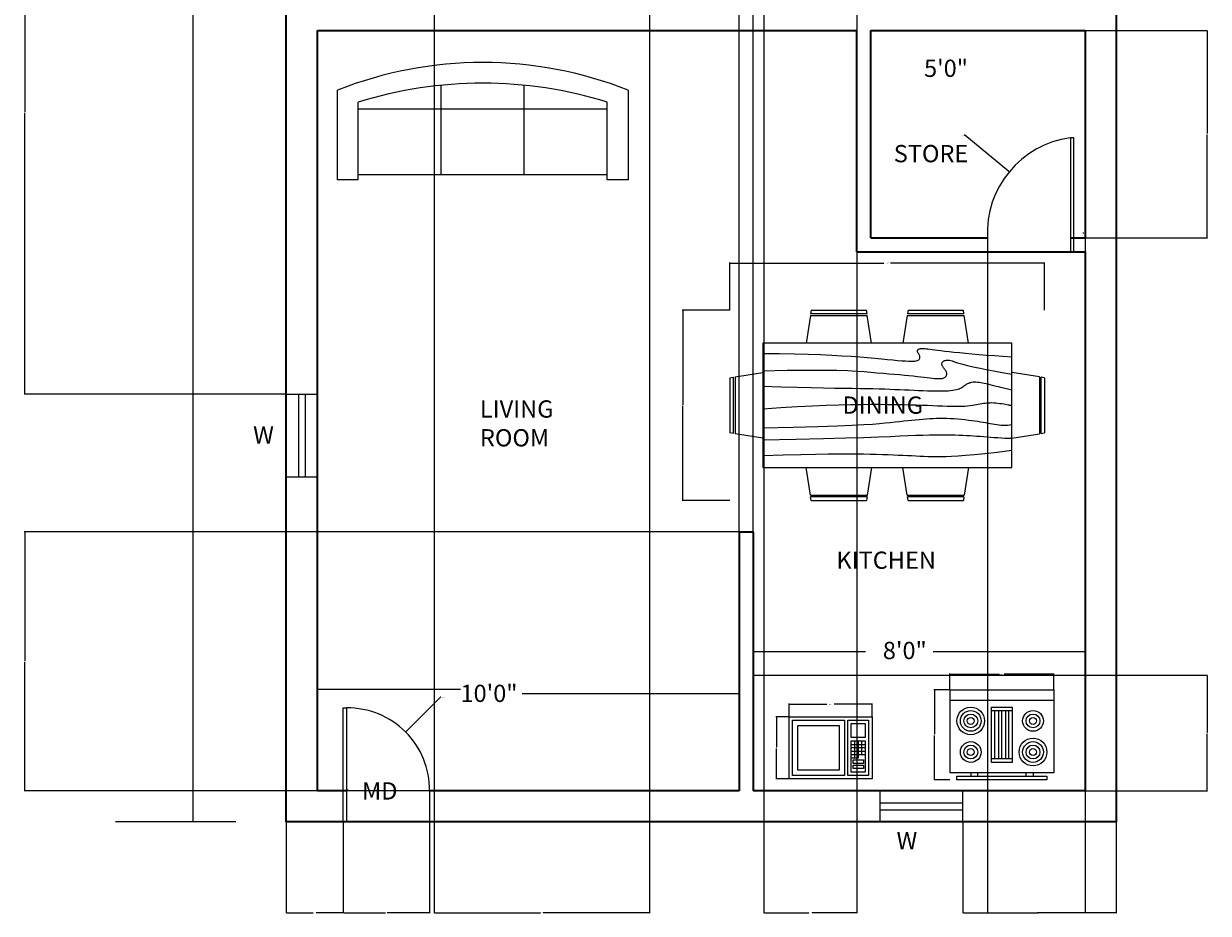
# Model space of a CAD drawing. Units: inches. Extents: x -58 to 719, y -488 to 73.
# Tile 1 of 3: x -58 to 284, y -488 to -231. Entities that reach past the tile are written whole.
import ezdxf

# ---------------------------------------------------------------- set-up
doc = ezdxf.new("R2010")
doc.units = ezdxf.units.IN
doc.header["$MEASUREMENT"] = 0
for name, color, linetype, lineweight in [('A-ANNO-DIMS', 2, 'Continuous', 13), ('A-ANNO-TEXT', 7, 'Continuous', 18), ('A-AREA-IDEN', 7, 'Continuous', 25), ('A-DOOR', 3, 'Continuous', 25), ('A-EQPM', 8, 'Continuous', 18), ('A-FLOR-CASE', 8, 'Continuous', 25), ('A-FURN', 8, 'Continuous', 18), ('A-GLAZ', 4, 'Continuous', 18), ('A-WALL', 7, 'Continuous', 35)]:
    doc.layers.add(name, color=color, linetype=linetype, lineweight=lineweight)
doc.styles.get("Standard").update_dxf_attribs({"font": 'arial.ttf'})
doc.dimstyles.get("Standard").update_dxf_attribs({"dimtxt": 0.18, "dimasz": 0.18, "dimexe": 0.18, "dimexo": 0.0625, "dimgap": 0.09, "dimtad": 0, "dimtih": 1, "dimtoh": 1, "dimdec": 4, "dimzin": 0, "dimdsep": 46, "dimtxsty": 'Standard', "dimcen": 0.09, "dimadec": 0, "dimazin": 0, "dimtfac": 1, "dimtdec": 4, "dimtofl": 0, "dimtmove": 0, "dimatfit": 3, "dimfxl": 1, "dimtolj": 1, "dimtzin": 0, "dimarcsym": 0})

# ---------------------------------------------------------------- blocks, each defined once
blk = doc.blocks.new('Dining Set - 36 x 72 in.')
for p, q in [((-22, 27.5), (-22.1562, 26.50042)), ((-22, 27.5), (-6, 27.5)), ((-5.8437, 26.49966), (-6, 27.5)), ((6, 27.5), (5.8438, 26.50042)), ((6, 27.5), (22, 27.5)), ((22.1563, 26.49966), (22, 27.5)), ((-22.2343, 26.00059), (-23.4847, 17.99762)), ((-22.2304, 26), (-5.7608, 26)), ((-5.8416, 26.5), (-22.1534, 26.5)), ((-4.5152, 17.99762), (-5.7655, 25.99926)), ((5.7657, 26.00059), (4.5153, 17.99762)), ((5.7696, 26), (22.2392, 26)), ((22.1584, 26.5), (5.8466, 26.5)), ((23.4848, 17.99762), (22.2345, 25.99926)), ((36, 18), (-36, 18)), ((-36, 18), (-36, -18)), ((36, -18), (36, 18)), ((-45.5, 8), (-44.5004, 8.15617)), ((-45.5, 8), (-45.5, -8)), ((-44.5, -8.15843), (-44.5, 8.15338)), ((-44.0006, 8.23428), (-35.9976, 9.48474)), ((-44, 8.23041), (-44, -8.23915)), ((44.0006, 8.23428), (35.9976, 9.48474)), ((44, 8.23041), (44, -8.23915)), ((44.5, -8.15843), (44.5, 8.15338)), ((45.5, 8), (44.5005, 8.15617)), ((45.5, 8), (45.5, -8)), ((-44.4997, -8.15631), (-45.5, -8)), ((-35.9976, -9.48476), (-43.9993, -8.2345)), ((35.9976, -9.48476), (43.9993, -8.2345)), ((44.4997, -8.15631), (45.5, -8)), ((-36, -18), (36, -18)), ((-22.2343, -26.0006), (-23.4847, -17.99762)), ((-4.5152, -17.99762), (-5.7655, -25.99928)), ((5.7657, -26.0006), (4.5153, -17.99762)), ((23.4848, -17.99762), (22.2345, -25.99928)), ((-22.2304, -26), (-5.7608, -26)), ((-22, -27.5), (-22.1562, -26.50044)), ((-5.8416, -26.5), (-22.1534, -26.5)), ((-5.8437, -26.49967), (-6, -27.5)), ((5.7696, -26), (22.2392, -26)), ((6, -27.5), (5.8438, -26.50044)), ((22.1584, -26.5), (5.8466, -26.5)), ((22.1563, -26.49967), (22, -27.5)), ((-22, -27.5), (-6, -27.5)), ((6, -27.5), (22, -27.5))]:
    blk.add_line(p, q)
for points in [[(-36, 15), (-31.1772, 14.97754), (-26.8079, 14.91406), (-22.8538, 14.81543), (-19.276, 14.6875), (-16.0362, 14.53613), (-13.0957, 14.36718), (-10.4159, 14.18652), (-7.9583, 14), (-5.6904, 13.81315), (-3.6035, 13.63021), (-1.6954, 13.45508), (0.0365, 13.29166), (1.5945, 13.14388), (2.9811, 13.01562), (4.1988, 12.9108), (5.25, 12.83333), (6.1393, 12.78613), (6.8802, 12.76823), (7.4883, 12.77767), (7.9792, 12.8125), (8.3685, 12.87077), (8.6719, 12.95052), (8.9049, 13.0498), (9.0833, 13.16666), (9.2205, 13.29899), (9.3216, 13.44401), (9.3895, 13.59879), (9.4271, 13.76041), (9.4373, 13.92594), (9.4232, 14.09245), (9.3875, 14.257), (9.3333, 14.41666), (9.2638, 14.56917), (9.1836, 14.71484), (9.0975, 14.85465), (9.0104, 14.98958), (8.9272, 15.1206), (8.8529, 15.2487), (8.7922, 15.37483), (8.75, 15.5), (8.7305, 15.62467), (8.7344, 15.74739), (8.7617, 15.86621), (8.8125, 15.97916), (8.8867, 16.08431), (8.9844, 16.17968), (9.1055, 16.26334), (9.25, 16.33333), (9.4189, 16.38802), (9.6172, 16.42708), (9.8506, 16.45052), (10.125, 16.45833), (10.4463, 16.45052), (10.8203, 16.42708), (11.2529, 16.38802), (11.75, 16.33333), (12.3184, 16.26318), (12.9694, 16.17838), (13.7151, 16.07991), (14.5677, 15.96875), (15.5395, 15.84586), (16.6426, 15.71224), (17.8893, 15.56884), (19.2917, 15.41666), (20.859, 15.25667), (22.5879, 15.08984), (24.4721, 14.91715), (26.5052, 14.73958), (28.6809, 14.5581), (30.9929, 14.3737), (33.4347, 14.18733), (36, 14)], [(-36, 10), (-28.9766, 10.14274), (-23.1725, 10.20442), (-18.4241, 10.19775), (-14.5677, 10.13541), (-11.4399, 10.03011), (-8.877, 9.89453), (-6.7154, 9.74137), (-4.7917, 9.58333), (-2.9698, 9.43082), (-1.2246, 9.28515), (0.4415, 9.14534), (2.026, 9.01041), (3.5266, 8.87939), (4.9408, 8.7513), (6.266, 8.62516), (7.5, 8.5), (8.6411, 8.37549), (9.6914, 8.2539), (10.6538, 8.13818), (11.5312, 8.03125), (12.3267, 7.93603), (13.043, 7.85547), (13.6831, 7.79248), (14.25, 7.75), (14.7471, 7.7303), (15.1797, 7.73307), (15.5537, 7.75732), (15.875, 7.80208), (16.1494, 7.86637), (16.3828, 7.94922), (16.5811, 8.04964), (16.75, 8.16666), (16.8944, 8.29915), (17.0143, 8.44531), (17.1089, 8.60319), (17.1771, 8.77083), (17.218, 8.94629), (17.2305, 9.1276), (17.2137, 9.31282), (17.1667, 9.5), (17.0895, 9.6875), (16.987, 9.875), (16.8649, 10.0625), (16.7292, 10.25), (16.5856, 10.4375), (16.4401, 10.625), (16.2985, 10.8125), (16.1667, 11), (16.05, 11.18733), (15.9518, 11.3737), (15.8752, 11.5581), (15.8229, 11.73958), (15.798, 11.91715), (15.8034, 12.08984), (15.842, 12.25667), (15.9167, 12.41666), (16.0295, 12.56836), (16.1784, 12.70833), (16.3605, 12.83268), (16.5729, 12.9375), (16.8127, 13.01888), (17.0768, 13.07291), (17.3625, 13.0957), (17.6667, 13.08333), (17.9894, 13.03312), (18.3418, 12.94726), (18.7382, 12.82918), (19.1927, 12.68229), (19.7195, 12.51001), (20.3327, 12.31575), (21.0465, 12.10294), (21.875, 11.875), (22.8357, 11.63354), (23.959, 11.37304), (25.2786, 11.08618), (26.8282, 10.76562), (28.6414, 10.40405), (30.752, 9.99414), (33.1936, 9.52856), (36, 9)], [(-36, 5.5), (-30.7157, 5.3348), (-26.069, 5.20963), (-21.9946, 5.11767), (-18.4271, 5.05208), (-15.3009, 5.00602), (-12.5508, 4.97265), (-10.1112, 4.94515), (-7.9167, 4.91666), (-5.909, 4.88167), (-4.0586, 4.83984), (-2.3429, 4.79215), (-0.7396, 4.73958), (0.7739, 4.6831), (2.22, 4.6237), (3.6213, 4.56233), (5, 4.5), (6.373, 4.43782), (7.7344, 4.3776), (9.0723, 4.32129), (10.375, 4.27083), (11.6309, 4.22819), (12.8281, 4.19531), (13.9551, 4.17415), (15, 4.16666), (15.954, 4.17448), (16.819, 4.19791), (17.6001, 4.23698), (18.3021, 4.29166), (18.9299, 4.36198), (19.4883, 4.44791), (19.9823, 4.54948), (20.4167, 4.66666), (20.7969, 4.79899), (21.1302, 4.94401), (21.4245, 5.09879), (21.6875, 5.26041), (21.9271, 5.42594), (22.1511, 5.59245), (22.3672, 5.757), (22.5834, 5.91666), (22.8065, 6.06868), (23.0404, 6.21093), (23.2879, 6.34147), (23.5521, 6.45833), (23.8358, 6.55957), (24.142, 6.64323), (24.4735, 6.70735), (24.8334, 6.75), (25.2235, 6.76969), (25.642, 6.76692), (26.0858, 6.74267), (26.5521, 6.69791), (27.0379, 6.63362), (27.5404, 6.55078), (28.0565, 6.45036), (28.5834, 6.33333), (29.1242, 6.19987), (29.7071, 6.04687), (30.3661, 5.87044), (31.1354, 5.66666), (32.0493, 5.43164), (33.142, 5.16146), (34.4475, 4.85221), (36, 4.5)], [(-36, -1), (-30.7915, -0.6591), (-26.0195, -0.38216), (-21.6519, -0.16284), (-17.6563, 0.00521), (-14.0005, 0.12833), (-10.6523, 0.21289), (-7.5796, 0.26522), (-4.75, 0.29166), (-2.134, 0.29793), (0.2878, 0.28711), (2.5317, 0.26163), (4.6146, 0.22396), (6.5529, 0.17651), (8.3633, 0.12174), (10.0623, 0.06209), (11.6667, 0), (13.1899, -0.06201), (14.6341, -0.1211), (15.9982, -0.17432), (17.2813, -0.21875), (18.4823, -0.25147), (19.6003, -0.26953), (20.6343, -0.27002), (21.5834, -0.25), (22.4481, -0.20768), (23.2357, -0.14584), (23.9549, -0.06836), (24.6146, 0.02083), (25.2235, 0.11784), (25.7904, 0.21875), (26.3241, 0.31966), (26.8334, 0.41666), (27.3265, 0.50618), (27.8099, 0.58593), (28.2894, 0.65397), (28.7709, 0.70833), (29.2601, 0.74707), (29.763, 0.76823), (30.2855, 0.76985), (30.8334, 0.75), (31.4088, 0.70784), (31.9994, 0.64713), (32.589, 0.57275), (33.1615, 0.48958), (33.7008, 0.4025), (34.1908, 0.3164), (34.6153, 0.23616), (34.9584, 0.16666), (35.2099, 0.11165), (35.3848, 0.07031), (35.504, 0.04069), (35.5886, 0.02083), (35.6594, 0.00879), (35.7377, 0.0026), (35.8442, 0.00032), (36, 0)], [(-36, -6.5), (-27.1843, -6.31267), (-20.084, -6.1263), (-14.469, -5.9419), (-10.1094, -5.76042), (-6.7752, -5.58285), (-4.2363, -5.41016), (-2.2629, -5.24333), (-0.625, -5.08334), (0.8708, -4.93099), (2.2715, -4.78646), (3.5872, -4.64974), (4.8281, -4.52084), (6.0046, -4.39974), (7.127, -4.28646), (8.2053, -4.18099), (9.25, -4.08334), (10.2705, -3.99382), (11.2734, -3.91407), (12.2647, -3.84603), (13.25, -3.79167), (14.2354, -3.75293), (15.2266, -3.73177), (16.2295, -3.73015), (17.25, -3.75), (18.2912, -3.79248), (19.3451, -3.85547), (20.4009, -3.93604), (21.4479, -4.03125), (22.4754, -4.13819), (23.4727, -4.25391), (24.4289, -4.37549), (25.3334, -4.5), (26.1785, -4.62492), (26.9694, -4.74935), (27.7145, -4.87281), (28.4219, -4.99479), (29.1, -5.11483), (29.7572, -5.23242), (30.4016, -5.34709), (31.0417, -5.45834), (31.6837, -5.56437), (32.3262, -5.65821), (32.9658, -5.73153), (33.599, -5.77604), (34.2224, -5.78345), (34.8327, -5.74545), (35.4264, -5.65373), (36, -5.5)], [(-36, -10), (-26.4022, -9.81299), (-18.4675, -9.62891), (-11.9839, -9.45069), (-6.7396, -9.28125), (-2.5226, -9.12354), (0.8789, -8.98047), (3.6769, -8.85498), (6.0833, -8.75), (8.2767, -8.66765), (10.3021, -8.60677), (12.1712, -8.56543), (13.8958, -8.54167), (15.4876, -8.53353), (16.9583, -8.53907), (18.3197, -8.55632), (19.5834, -8.58334), (20.7616, -8.61841), (21.8685, -8.66081), (22.9188, -8.71004), (23.9271, -8.76563), (24.9081, -8.82707), (25.8763, -8.89388), (26.8465, -8.96558), (27.8334, -9.04167), (28.8474, -9.12118), (29.8828, -9.20117), (30.93, -9.27824), (31.9792, -9.34896), (33.0205, -9.40991), (34.0443, -9.45768), (35.0407, -9.48885), (36, -9.5)], [(-36, -14.5), (-30.0881, -14.33513), (-25.0332, -14.21224), (-20.7312, -14.12647), (-17.0781, -14.07292), (-13.97, -14.04671), (-11.3027, -14.04297), (-8.9724, -14.05681), (-6.875, -14.08334), (-4.9224, -14.11833), (-3.0905, -14.16016), (-1.3709, -14.20785), (0.2448, -14.26042), (1.7647, -14.3169), (3.1973, -14.3763), (4.5507, -14.43767), (5.8333, -14.5), (7.0554, -14.5621), (8.235, -14.62175), (9.3922, -14.67652), (10.5469, -14.72396), (11.7192, -14.76164), (12.929, -14.78711), (14.1965, -14.79794), (15.5417, -14.79167), (16.9933, -14.76424), (18.6152, -14.70508), (20.4804, -14.60197), (22.6615, -14.44271), (25.2312, -14.21509), (28.2624, -13.9069), (31.8277, -13.50594), (36, -13)]]:
    blk.add_lwpolyline(points)
blk = doc.blocks.new('Range-Oven - 30 in top')
for p, q in [((0, -3), (30, -3)), ((12, -6), (18, -6)), ((13, -20), (13, -6)), ((14, -6), (14, -20)), ((15, -20), (15, -6)), ((16, -6), (16, -20)), ((17, -20), (17, -6)), ((18, -20), (12, -20)), ((6, -24), (6, -25)), ((8, -25), (8, -24)), ((22, -25), (22, -24)), ((24, -24), (24, -25))]:
    blk.add_line(p, q)
for points in [[(0, -24), (0, 0), (30, 0), (30, -24)], [(12, -21), (12, -5), (18, -5), (18, -21)], [(2, -26), (2, -25), (28, -25), (28, -26)]]:
    blk.add_lwpolyline(points, close=True)
for centre, radius in [((6, -9), 4), ((6, -9), 3), ((24, -9), 3), ((6, -9), 2), ((6, -9), 1), ((24, -9), 2), ((24, -9), 1), ((6, -18), 3), ((6, -18), 2), ((6, -18), 1), ((24, -18), 4), ((24, -18), 3), ((24, -18), 2), ((24, -18), 1)]:
    blk.add_circle(centre, radius)
blk = doc.blocks.new('Microwave')
for p, q in [((19, 7), (19, 11)), ((20, 11), (20, 7)), ((21, 7), (21, 11)), ((18, 10), (22, 10)), ((22, 9), (18, 9)), ((18, 8), (22, 8)), ((22, 7), (18, 7)), ((19, 6), (19, 7)), ((20, 7), (20, 6)), ((20, 6), (18, 6))]:
    blk.add_line(p, q)
for points in [[(0, 0), (0, 18), (24, 18), (24, 0)], [(1, 1), (1, 17), (16, 17), (16, 1)], [(2.5, 2.5), (2.5, 15.5), (14.5, 15.5), (14.5, 2.5)], [(17, 1), (17, 17), (23, 17), (23, 1)], [(18, 12), (18, 16), (22, 16), (22, 12)], [(18, 2), (18, 11), (22, 11), (22, 2)], [(18.5, 4.5), (18.5, 5.5), (21.5, 5.5), (21.5, 4.5)], [(18.5, 3), (18.5, 4), (21.5, 4), (21.5, 3)]]:
    blk.add_lwpolyline(points, close=True)
blk = doc.blocks.new('Sofa - Roundback 7 ft.')
for p, q in [((-12.00002, -32.4421), (-12.00003, -6.5971)), ((11.99997, -32.4421), (11.99998, -6.5971)), ((-36.000027, -34), (-36.000027, -11.4696)), ((-35.999844, -13.3819), (35.9998, -13.3819)), ((35.99998, -34), (35.99998, -11.4696)), ((-36.000027, -32.4421), (35.99998, -32.4421))]:
    blk.add_line(p, q)
for points in [[(-36.000027, -34), (-42.000027, -34), (-42.000027, -8)], [(41.99998, -8), (41.99998, -34), (35.99998, -34)]]:
    blk.add_lwpolyline(points)
for centre, radius, start, end in [((0, -114.25), 114.25, 68.43141, 111.5686), ((-0.00001, -127.1968), 121.1968, 72.72033, 107.2797)]:
    blk.add_arc(centre, radius, start, end)
blk = doc.blocks.new('WIN-24IN')
for p, q in [((3.5, 24), (3.5, 0)), ((5.5, 24), (5.5, 0))]:
    blk.add_line(p, q)
blk.add_lwpolyline([(0, 24), (9, 24), (9, 0), (0, 0)], close=True)
blk = doc.blocks.new('*D19')
at = {"layer": 'A-ANNO-DIMS', "color": 0, "lineweight": -2, "transparency": 16777216}
for p, q in [((145.9, -313.4), (145.9, -299.63)), ((146.08, -299.81), (190.45, -299.81)), ((236.72, -299.81), (192.35, -299.81)), ((236.9, -313.4), (236.9, -299.63))]:
    blk.add_line(p, q, dxfattribs=at)
at = {"layer": 'A-ANNO-DIMS', "color": 0, "transparency": 16777216}
for points in [[(146.08, -299.78), (146.08, -299.84), (145.9, -299.81)], [(236.72, -299.78), (236.72, -299.84), (236.9, -299.81)]]:
    blk.add_solid(points, dxfattribs=at)
at = {"layer": 'Defpoints', "color": 0, "transparency": 16777216}
for p in [(236.9, -299.81), (145.9, -313.46), (236.9, -313.46)]:
    blk.add_point(p, dxfattribs=at)
at = {"layer": 'A-ANNO-DIMS', "color": 0, "transparency": 16777216, "insert": (191.4, -299.81), "char_height": 0.18, "attachment_point": 5}
blk.add_mtext('\\A1;DINING SET 91', dxfattribs=at)
blk = doc.blocks.new('*D20')
at = {"layer": 'A-ANNO-DIMS', "color": 0, "lineweight": -2, "transparency": 16777216}
for p, q in [((145.84, -313.46), (132.07, -313.46)), ((132.25, -313.64), (132.25, -340.78)), ((132.25, -368.28), (132.25, -341.14)), ((145.84, -368.46), (132.07, -368.46))]:
    blk.add_line(p, q, dxfattribs=at)
at = {"layer": 'A-ANNO-DIMS', "color": 0, "transparency": 16777216}
for points in [[(132.22, -313.64), (132.28, -313.64), (132.25, -313.46)], [(132.22, -368.28), (132.28, -368.28), (132.25, -368.46)]]:
    blk.add_solid(points, dxfattribs=at)
at = {"layer": 'Defpoints', "color": 0, "transparency": 16777216}
for p in [(132.25, -313.46), (145.9, -313.46), (145.9, -368.46)]:
    blk.add_point(p, dxfattribs=at)
at = {"layer": 'A-ANNO-DIMS', "color": 0, "transparency": 16777216, "insert": (132.25, -340.96), "char_height": 0.18, "attachment_point": 5}
blk.add_mtext('\\A1;55', dxfattribs=at)
blk = doc.blocks.new('*D21')
at = {"layer": 'A-ANNO-DIMS', "color": 0, "lineweight": -2, "transparency": 16777216}
for p, q in [((209.54, -423.22), (209.54, -418.6)), ((209.72, -418.78), (223.85, -418.78)), ((239.36, -418.78), (225.24, -418.78)), ((239.54, -423.22), (239.54, -418.6))]:
    blk.add_line(p, q, dxfattribs=at)
at = {"layer": 'A-ANNO-DIMS', "color": 0, "transparency": 16777216}
for points in [[(209.72, -418.75), (209.72, -418.81), (209.54, -418.78)], [(239.36, -418.75), (239.36, -418.81), (239.54, -418.78)]]:
    blk.add_solid(points, dxfattribs=at)
at = {"layer": 'Defpoints', "color": 0, "transparency": 16777216}
for p in [(239.54, -418.78), (209.54, -423.28), (239.54, -423.28)]:
    blk.add_point(p, dxfattribs=at)
at = {"layer": 'A-ANNO-DIMS', "color": 0, "transparency": 16777216, "insert": (224.54, -418.78), "char_height": 0.18, "attachment_point": 5}
blk.add_mtext('\\A1;RANGE 30', dxfattribs=at)
blk = doc.blocks.new('*D22')
at = {"layer": 'A-ANNO-DIMS', "color": 0, "lineweight": -2, "transparency": 16777216}
for p, q in [((209.48, -423.28), (204.86, -423.28)), ((205.04, -423.46), (205.04, -436.1)), ((205.04, -449.1), (205.04, -436.46)), ((209.48, -449.28), (204.86, -449.28))]:
    blk.add_line(p, q, dxfattribs=at)
at = {"layer": 'A-ANNO-DIMS', "color": 0, "transparency": 16777216}
for points in [[(205.01, -423.46), (205.07, -423.46), (205.04, -423.28)], [(205.01, -449.1), (205.07, -449.1), (205.04, -449.28)]]:
    blk.add_solid(points, dxfattribs=at)
at = {"layer": 'Defpoints', "color": 0, "transparency": 16777216}
for p in [(205.04, -423.28), (209.54, -423.28), (209.54, -449.28)]:
    blk.add_point(p, dxfattribs=at)
at = {"layer": 'A-ANNO-DIMS', "color": 0, "transparency": 16777216, "insert": (205.04, -436.28), "char_height": 0.18, "attachment_point": 5}
blk.add_mtext('\\A1;26', dxfattribs=at)
blk = doc.blocks.new('*D23')
at = {"layer": 'A-ANNO-DIMS', "color": 0, "lineweight": -2, "transparency": 16777216}
for p, q in [((163, -431), (163, -427.28)), ((163.18, -427.46), (173.96, -427.46)), ((186.82, -427.46), (176.04, -427.46)), ((187, -431), (187, -427.28))]:
    blk.add_line(p, q, dxfattribs=at)
at = {"layer": 'A-ANNO-DIMS', "color": 0, "transparency": 16777216}
for points in [[(163.18, -427.43), (163.18, -427.49), (163, -427.46)], [(186.82, -427.43), (186.82, -427.49), (187, -427.46)]]:
    blk.add_solid(points, dxfattribs=at)
at = {"layer": 'Defpoints', "color": 0, "transparency": 16777216}
for p in [(187, -427.46), (163, -431.06), (187, -431.06)]:
    blk.add_point(p, dxfattribs=at)
at = {"layer": 'A-ANNO-DIMS', "color": 0, "transparency": 16777216, "insert": (175, -427.46), "char_height": 0.18, "attachment_point": 5}
blk.add_mtext('\\A1;MICROWAVE 24', dxfattribs=at)
blk = doc.blocks.new('*D24')
at = {"layer": 'A-ANNO-DIMS', "color": 0, "lineweight": -2, "transparency": 16777216}
for p, q in [((162.94, -431.06), (159.22, -431.06)), ((159.4, -431.24), (159.4, -439.88)), ((159.4, -448.88), (159.4, -440.25)), ((162.94, -449.06), (159.22, -449.06))]:
    blk.add_line(p, q, dxfattribs=at)
at = {"layer": 'A-ANNO-DIMS', "color": 0, "transparency": 16777216}
for points in [[(159.37, -431.24), (159.43, -431.24), (159.4, -431.06)], [(159.37, -448.88), (159.43, -448.88), (159.4, -449.06)]]:
    blk.add_solid(points, dxfattribs=at)
at = {"layer": 'Defpoints', "color": 0, "transparency": 16777216}
for p in [(159.4, -431.06), (163, -431.06), (163, -449.06)]:
    blk.add_point(p, dxfattribs=at)
at = {"layer": 'A-ANNO-DIMS', "color": 0, "transparency": 16777216, "insert": (159.4, -440.06), "char_height": 0.18, "attachment_point": 5}
blk.add_mtext('\\A1;18', dxfattribs=at)
blk = doc.blocks.new('*D25')
at = {"layer": 'A-ANNO-DIMS', "color": 0, "lineweight": -2, "transparency": 16777216}
for p, q in [((248.67, -232.52), (284.04, -232.52)), ((283.86, -232.7), (283.86, -262.34)), ((283.86, -292.34), (283.86, -262.7)), ((248.67, -292.52), (284.04, -292.52))]:
    blk.add_line(p, q, dxfattribs=at)
at = {"layer": 'A-ANNO-DIMS', "color": 0, "transparency": 16777216}
for points in [[(283.83, -232.7), (283.89, -232.7), (283.86, -232.52)], [(283.83, -292.34), (283.89, -292.34), (283.86, -292.52)]]:
    blk.add_solid(points, dxfattribs=at)
at = {"layer": 'Defpoints', "color": 0, "transparency": 16777216}
for p in [(248.61, -232.52), (248.61, -292.52), (283.86, -292.52)]:
    blk.add_point(p, dxfattribs=at)
at = {"layer": 'A-ANNO-DIMS', "color": 0, "transparency": 16777216, "insert": (283.86, -262.52), "char_height": 0.18, "attachment_point": 5}
blk.add_mtext('\\A1;60', dxfattribs=at)
blk = doc.blocks.new('*D26')
at = {"layer": 'A-ANNO-DIMS', "color": 0, "lineweight": -2, "transparency": 16777216}
for p, q in [((148.55, -377.58), (-58.2, -377.58)), ((-58.02, -377.76), (-58.02, -414.87)), ((-58.02, -452.34), (-58.02, -415.24)), ((148.55, -452.52), (-58.2, -452.52))]:
    blk.add_line(p, q, dxfattribs=at)
at = {"layer": 'A-ANNO-DIMS', "color": 0, "transparency": 16777216}
for points in [[(-58.05, -377.76), (-57.99, -377.76), (-58.02, -377.58)], [(-58.05, -452.34), (-57.99, -452.34), (-58.02, -452.52)]]:
    blk.add_solid(points, dxfattribs=at)
at = {"layer": 'Defpoints', "color": 0, "transparency": 16777216}
for p in [(148.61, -377.58), (-58.02, -452.52), (148.61, -452.52)]:
    blk.add_point(p, dxfattribs=at)
at = {"layer": 'A-ANNO-DIMS', "color": 0, "transparency": 16777216, "insert": (-58.02, -415.05), "char_height": 0.18, "attachment_point": 5}
blk.add_mtext('\\A1;74.94', dxfattribs=at)
blk = doc.blocks.new('*D27')
at = {"layer": 'A-ANNO-DIMS', "color": 0, "lineweight": -2, "transparency": 16777216}
for p, q in [((248.67, -419.05), (284.04, -419.05)), ((283.86, -419.23), (283.86, -435.6)), ((283.86, -452.34), (283.86, -435.97)), ((248.67, -452.52), (284.04, -452.52))]:
    blk.add_line(p, q, dxfattribs=at)
at = {"layer": 'A-ANNO-DIMS', "color": 0, "transparency": 16777216}
for points in [[(283.83, -419.23), (283.89, -419.23), (283.86, -419.05)], [(283.83, -452.34), (283.89, -452.34), (283.86, -452.52)]]:
    blk.add_solid(points, dxfattribs=at)
at = {"layer": 'Defpoints', "color": 0, "transparency": 16777216}
for p in [(248.61, -419.05), (248.61, -452.52), (283.86, -452.52)]:
    blk.add_point(p, dxfattribs=at)
at = {"layer": 'A-ANNO-DIMS', "color": 0, "transparency": 16777216, "insert": (283.86, -435.79), "char_height": 0.18, "attachment_point": 5}
blk.add_mtext('\\A1;33.475', dxfattribs=at)
blk = doc.blocks.new('*D30')
at = {"layer": 'A-ANNO-DIMS', "color": 0, "lineweight": -2, "transparency": 16777216}
for p, q in [((17.55, -174.83), (-58.2, -174.83)), ((-58.02, -175.01), (-58.02, -256.1)), ((-58.02, -337.55), (-58.02, -256.46)), ((17.55, -337.73), (-58.2, -337.73))]:
    blk.add_line(p, q, dxfattribs=at)
at = {"layer": 'A-ANNO-DIMS', "color": 0, "transparency": 16777216}
for points in [[(-58.05, -175.01), (-57.99, -175.01), (-58.02, -174.83)], [(-58.05, -337.55), (-57.99, -337.55), (-58.02, -337.73)]]:
    blk.add_solid(points, dxfattribs=at)
at = {"layer": 'Defpoints', "color": 0, "transparency": 16777216}
for p in [(17.61, -174.83), (-58.02, -337.73), (17.61, -337.73)]:
    blk.add_point(p, dxfattribs=at)
at = {"layer": 'A-ANNO-DIMS', "color": 0, "transparency": 16777216, "insert": (-58.02, -256.28), "char_height": 0.18, "attachment_point": 5}
blk.add_mtext('\\A1;162.9', dxfattribs=at)
blk = doc.blocks.new('*D38')
at = {"layer": 'A-ANNO-DIMS', "color": 0, "lineweight": -2, "transparency": 16777216}
for p, q in [((17.61, -461.59), (17.61, -487.95)), ((34.05, -461.59), (34.05, -487.95)), ((17.79, -487.77), (25.37, -487.77)), ((33.87, -487.77), (26.29, -487.77))]:
    blk.add_line(p, q, dxfattribs=at)
at = {"layer": 'A-ANNO-DIMS', "color": 0, "transparency": 16777216}
for points in [[(17.79, -487.74), (17.79, -487.8), (17.61, -487.77)], [(33.87, -487.74), (33.87, -487.8), (34.05, -487.77)]]:
    blk.add_solid(points, dxfattribs=at)
at = {"layer": 'Defpoints', "color": 0, "transparency": 16777216}
for p in [(17.61, -461.52), (34.05, -461.52), (34.05, -487.77)]:
    blk.add_point(p, dxfattribs=at)
at = {"layer": 'A-ANNO-DIMS', "color": 0, "transparency": 16777216, "insert": (25.83, -487.77), "char_height": 0.18, "attachment_point": 5}
blk.add_mtext('\\A1;16.435', dxfattribs=at)
blk = doc.blocks.new('*D39')
at = {"layer": 'A-ANNO-DIMS', "color": 0, "lineweight": -2, "transparency": 16777216}
for p, q in [((59.05, -452.59), (59.05, -487.95)), ((34.05, -461.59), (34.05, -487.95)), ((34.23, -487.77), (46.33, -487.77)), ((58.87, -487.77), (46.77, -487.77))]:
    blk.add_line(p, q, dxfattribs=at)
at = {"layer": 'A-ANNO-DIMS', "color": 0, "transparency": 16777216}
for points in [[(34.23, -487.74), (34.23, -487.8), (34.05, -487.77)], [(58.87, -487.74), (58.87, -487.8), (59.05, -487.77)]]:
    blk.add_solid(points, dxfattribs=at)
at = {"layer": 'Defpoints', "color": 0, "transparency": 16777216}
for p in [(59.05, -452.52), (34.05, -461.52), (59.05, -487.77)]:
    blk.add_point(p, dxfattribs=at)
at = {"layer": 'A-ANNO-DIMS', "color": 0, "transparency": 16777216, "insert": (46.55, -487.77), "char_height": 0.18, "attachment_point": 5}
blk.add_mtext('\\A1;25', dxfattribs=at)
blk = doc.blocks.new('*D40')
at = {"layer": 'A-ANNO-DIMS', "color": 0, "lineweight": -2, "transparency": 16777216}
for p, q in [((213.23, -461.59), (213.23, -487.95)), ((257.61, -461.59), (257.61, -487.95)), ((213.41, -487.77), (235.03, -487.77)), ((257.43, -487.77), (235.82, -487.77))]:
    blk.add_line(p, q, dxfattribs=at)
at = {"layer": 'A-ANNO-DIMS', "color": 0, "transparency": 16777216}
for points in [[(213.41, -487.74), (213.41, -487.8), (213.23, -487.77)], [(257.43, -487.74), (257.43, -487.8), (257.61, -487.77)]]:
    blk.add_solid(points, dxfattribs=at)
at = {"layer": 'Defpoints', "color": 0, "transparency": 16777216}
for p in [(213.23, -461.52), (257.61, -461.52), (257.61, -487.77)]:
    blk.add_point(p, dxfattribs=at)
at = {"layer": 'A-ANNO-DIMS', "color": 0, "transparency": 16777216, "insert": (235.42, -487.77), "char_height": 0.18, "attachment_point": 5}
blk.add_mtext('\\A1;44.38', dxfattribs=at)
blk = doc.blocks.new('*D43')
at = {"layer": 'A-ANNO-DIMS', "color": 0, "lineweight": -2, "transparency": 16777216}
for p, q in [((60.38, -153.59), (60.38, -487.95)), ((122.61, -153.59), (122.61, -487.95)), ((60.56, -487.77), (91.1, -487.77)), ((122.43, -487.77), (91.89, -487.77))]:
    blk.add_line(p, q, dxfattribs=at)
at = {"layer": 'A-ANNO-DIMS', "color": 0, "transparency": 16777216}
for points in [[(60.56, -487.74), (60.56, -487.8), (60.38, -487.77)], [(122.43, -487.74), (122.43, -487.8), (122.61, -487.77)]]:
    blk.add_solid(points, dxfattribs=at)
at = {"layer": 'Defpoints', "color": 0, "transparency": 16777216}
for p in [(60.38, -153.52), (122.61, -153.52), (122.61, -487.77)]:
    blk.add_point(p, dxfattribs=at)
at = {"layer": 'A-ANNO-DIMS', "color": 0, "transparency": 16777216, "insert": (91.5, -487.77), "char_height": 0.18, "attachment_point": 5}
blk.add_mtext('\\A1;62.23', dxfattribs=at)
blk = doc.blocks.new('*D49')
at = {"layer": 'A-ANNO-DIMS', "color": 0, "lineweight": -2, "transparency": 16777216}
for p, q in [((155.75, -122.59), (155.75, -487.95)), ((182.61, -122.59), (182.61, -487.95)), ((155.93, -487.77), (168.71, -487.77)), ((182.43, -487.77), (169.64, -487.77))]:
    blk.add_line(p, q, dxfattribs=at)
at = {"layer": 'A-ANNO-DIMS', "color": 0, "transparency": 16777216}
for points in [[(155.93, -487.74), (155.93, -487.8), (155.75, -487.77)], [(182.43, -487.74), (182.43, -487.8), (182.61, -487.77)]]:
    blk.add_solid(points, dxfattribs=at)
at = {"layer": 'Defpoints', "color": 0, "transparency": 16777216}
for p in [(155.75, -122.52), (182.61, -122.52), (182.61, -487.77)]:
    blk.add_point(p, dxfattribs=at)
at = {"layer": 'A-ANNO-DIMS', "color": 0, "transparency": 16777216, "insert": (169.18, -487.77), "char_height": 0.18, "attachment_point": 5}
blk.add_mtext('\\A1;26.867', dxfattribs=at)
blk = doc.blocks.new('*D52')
at = {"layer": 'A-ANNO-DIMS', "color": 0, "lineweight": -2, "transparency": 16777216}
for p, q in [((220.35, -292.59), (220.35, -487.95)), ((248.61, -292.59), (248.61, -487.95)), ((220.53, -487.77), (234.09, -487.77)), ((248.43, -487.77), (234.88, -487.77))]:
    blk.add_line(p, q, dxfattribs=at)
at = {"layer": 'A-ANNO-DIMS', "color": 0, "transparency": 16777216}
for points in [[(220.53, -487.74), (220.53, -487.8), (220.35, -487.77)], [(248.43, -487.74), (248.43, -487.8), (248.61, -487.77)]]:
    blk.add_solid(points, dxfattribs=at)
at = {"layer": 'Defpoints', "color": 0, "transparency": 16777216}
for p in [(220.35, -292.52), (248.61, -292.52), (248.61, -487.77)]:
    blk.add_point(p, dxfattribs=at)
at = {"layer": 'A-ANNO-DIMS', "color": 0, "transparency": 16777216, "insert": (234.48, -487.77), "char_height": 0.18, "attachment_point": 5}
blk.add_mtext('\\A1;28.26', dxfattribs=at)
blk = doc.blocks.new('*D57')
at = {"layer": 'A-ANNO-DIMS', "color": 0, "lineweight": -2, "transparency": 16777216}
for p, q in [((148.61, -377.52), (148.61, 73.06)), ((148.79, 72.88), (150.46, 72.88)), ((152.43, 72.88), (150.76, 72.88)), ((152.61, -377.52), (152.61, 73.06))]:
    blk.add_line(p, q, dxfattribs=at)
at = {"layer": 'A-ANNO-DIMS', "color": 0, "transparency": 16777216}
for points in [[(148.79, 72.91), (148.79, 72.85), (148.61, 72.88)], [(152.43, 72.91), (152.43, 72.85), (152.61, 72.88)]]:
    blk.add_solid(points, dxfattribs=at)
at = {"layer": 'Defpoints', "color": 0, "transparency": 16777216}
for p in [(152.61, 72.88), (148.61, -377.58), (152.61, -377.58)]:
    blk.add_point(p, dxfattribs=at)
at = {"layer": 'A-ANNO-DIMS', "color": 0, "transparency": 16777216, "insert": (150.61, 72.88), "char_height": 0.18, "attachment_point": 5}
blk.add_mtext('\\A1;4', dxfattribs=at)
blk = doc.blocks.new('*D59')
at = {"layer": 'A-ANNO-DIMS', "color": 0, "lineweight": -2, "transparency": 16777216}
for p, q in [((62.16, -425.41), (52.24, -435.33)), ((62.34, -425.41), (62.16, -425.41)), ((35.37, -452.29), (35.37, -452.11)), ((35.28, -452.2), (35.46, -452.2))]:
    blk.add_line(p, q, dxfattribs=at)
at = {"layer": 'A-ANNO-DIMS', "color": 0, "transparency": 16777216}
blk.add_solid([(52.22, -435.31), (52.26, -435.35), (52.11, -435.46)], dxfattribs=at)
at = {"layer": 'Defpoints', "color": 0, "transparency": 16777216}
for p in [(52.11, -435.46), (35.37, -452.2)]:
    blk.add_point(p, dxfattribs=at)
at = {"layer": 'A-ANNO-DIMS', "color": 0, "transparency": 16777216, "insert": (62.89, -425.41), "char_height": 0.18, "attachment_point": 5}
blk.add_mtext('\\A1;R23.683', dxfattribs=at)
blk = doc.blocks.new('*D63')
at = {"layer": 'A-ANNO-DIMS', "color": 0, "lineweight": -2, "transparency": 16777216}
for p, q in [((213.67, -262.71), (213.85, -262.71)), ((213.85, -262.71), (226.57, -273.23)), ((248.04, -291.08), (248.22, -291.08)), ((248.13, -291.17), (248.13, -290.99))]:
    blk.add_line(p, q, dxfattribs=at)
at = {"layer": 'A-ANNO-DIMS', "color": 0, "transparency": 16777216}
blk.add_solid([(226.58, -273.21), (226.55, -273.26), (226.7, -273.35)], dxfattribs=at)
at = {"layer": 'Defpoints', "color": 0, "transparency": 16777216}
for p in [(226.7, -273.35), (248.13, -291.08)]:
    blk.add_point(p, dxfattribs=at)
at = {"layer": 'A-ANNO-DIMS', "color": 0, "transparency": 16777216, "insert": (213.12, -262.71), "char_height": 0.18, "attachment_point": 5}
blk.add_mtext('\\A1;R27.816', dxfattribs=at)

msp = doc.modelspace()

# ---------------------------------------------------------------- linework, layer by layer
at = {"layer": 'A-ANNO-DIMS'}
for p, q in [((-9.4506, -208.4652), (-9.4506, -461.523)), ((152.6125, -412.1983), (185.062, -412.1983)), ((204.7154, -412.1983), (248.6125, -412.1983)), ((26.6125, -423.1239), (67.9788, -423.1239)), ((85.7824, -424.3357), (148.6125, -424.3357)), ((3.0224, -461.523), (-31.7687, -461.523))]:
    msp.add_line(p, q, dxfattribs=at)
at = {"layer": 'A-DOOR'}
for p, q in [((245.3548, -263.523), (244.3548, -263.523)), ((244.3548, -263.523), (244.3548, -296.523)), ((245.3548, -296.523), (245.3548, -263.523)), ((220.3548, -292.523), (220.3548, -296.523)), ((34.0475, -461.523), (34.0475, -428.523)), ((34.0475, -428.523), (35.0475, -428.523)), ((35.0475, -428.523), (35.0475, -461.523)), ((59.0475, -452.523), (59.0475, -461.523))]:
    msp.add_line(p, q, dxfattribs=at)
for centre, radius, start, end in [((248.1332, -291.081), 27.8159, 97.807081, 182.971543), ((35.3662, -452.2043), 23.6834, 359.228909, 90.771091)]:
    msp.add_arc(centre, radius, start, end, dxfattribs=at)
at = {"layer": 'A-FLOR-CASE'}
msp.add_line((152.6125, -419.0481), (248.6125, -419.0481), dxfattribs=at)
at = {"layer": 'A-WALL'}
for p, q in [((26.6125, -452.523), (26.6125, -232.523)), ((26.6125, -232.523), (182.6125, -232.523)), ((182.6125, -296.523), (182.6125, -232.523)), ((186.6125, -292.523), (186.6125, -232.523)), ((186.6125, -232.523), (248.6125, -232.523)), ((248.6125, -232.523), (248.6125, -292.523)), ((186.6125, -292.523), (220.3548, -292.523)), ((244.3548, -292.523), (248.6125, -292.523)), ((182.6125, -296.523), (248.6125, -296.523)), ((248.6125, -296.523), (248.6125, -452.523)), ((148.6125, -377.5847), (152.6125, -377.5847)), ((148.6125, -377.5847), (148.6125, -452.523)), ((152.6125, -377.5847), (152.6125, -452.523)), ((35.0475, -452.523), (26.6125, -452.523)), ((148.6125, -452.523), (59.0475, -452.523)), ((248.6125, -452.523), (152.6125, -452.523))]:
    msp.add_line(p, q, dxfattribs=at)
msp.add_lwpolyline([(17.6125, 18.477), (257.6125, 18.477), (257.6125, -461.523), (17.6125, -461.523)], close=True, dxfattribs=at)

# ---------------------------------------------------------------- block references
at = {"layer": 'A-EQPM'}
for name, p in [('Range-Oven - 30 in top', (209.5443, -423.2811)), ('Microwave', (162.9988, -449.064))]:
    msp.add_blockref(name, p, dxfattribs=at)
at = {"layer": 'A-FURN'}
for name, p in [('Sofa - Roundback 7 ft.', (74.4382, -241.7565)), ('Dining Set - 36 x 72 in.', (191.3977, -340.9579))]:
    msp.add_blockref(name, p, dxfattribs=at)
at = {"layer": 'A-GLAZ'}
msp.add_blockref('WIN-24IN', (17.612, -361.7265), dxfattribs=at)
at = {"layer": 'A-GLAZ', "extrusion": (0, 0, -1), "zscale": -1, "rotation": 270.0000000000001}
msp.add_blockref('WIN-24IN', (-213.2344, -452.5225), dxfattribs=at)

# ---------------------------------------------------------------- texts
at = {"layer": 'A-ANNO-DIMS', "char_height": 5, "attachment_point": 1}
for s, width, insert in [('5\'0"', 16.357695, (202.0286, -240.9287)), ('8\'0"', 14.09613, (190.1143, -409.399)), ('10\'0"', 35.99602, (67.9788, -421.8046))]:
    msp.add_mtext_dynamic_manual_height_columns(s, width=width, gutter_width=25, heights=[0], dxfattribs=dict(at, insert=insert))
at = {"layer": 'A-ANNO-TEXT', "char_height": 5, "attachment_point": 1}
for s, width, insert in [('W', 9.843431, (8.0278, -347.0456)), ('MD', 10.466109, (39.524, -450.0388)), ('W', 16.703304, (194.0832, -464.3989))]:
    msp.add_mtext_dynamic_manual_height_columns(s, width=width, gutter_width=25, heights=[0], dxfattribs=dict(at, insert=insert))
at = {"layer": 'A-AREA-IDEN', "char_height": 5, "attachment_point": 1}
for s, width, insert in [('STORE', 19.400991, (193.2792, -265.6265)), ('DINING', 31.211709, (178.4602, -338.397)), ('LIVING \\PROOM', 49.370331, (73.6101, -339.519)), ('KITCHEN', 53.537408, (176.705, -383.2684))]:
    msp.add_mtext_dynamic_manual_height_columns(s, width=width, gutter_width=25, heights=[0], dxfattribs=dict(at, insert=insert))

# ---------------------------------------------------------------- dimensions: what is measured, and where the dimension line sits
at = {"layer": 'A-ANNO-DIMS'}
for base, p1, p2, override, picture, middle in [((152.6125, 72.8793), (148.6125, -377.5847), (152.6125, -377.5847), {"dimdec": 0, "dimlfac": 1, "dimrnd": 0, "dimzin": 0, "dimdsep": 46, "dimlunit": 2}, '*D57', (150.6125, 72.8793)), ((182.6125, -487.773), (155.7455, -122.523), (182.6125, -122.523), {"dimdec": 3, "dimlfac": 1, "dimrnd": 0, "dimzin": 0, "dimdsep": 46, "dimlunit": 2}, '*D49', (169.179, -487.773)), ((122.6125, -487.773), (60.3821, -153.523), (122.6125, -153.523), {"dimdec": 2, "dimlfac": 1, "dimrnd": 0, "dimzin": 0, "dimdsep": 46, "dimlunit": 2}, '*D43', (91.4973, -487.773)), ((248.6125, -487.773), (220.3548, -292.523), (248.6125, -292.523), {"dimdec": 2, "dimlfac": 1, "dimrnd": 0, "dimzin": 0, "dimdsep": 46, "dimlunit": 2}, '*D52', (234.4836, -487.773)), ((59.0475, -487.773), (34.0475, -461.523), (59.0475, -452.523), {"dimdec": 0, "dimlfac": 1, "dimrnd": 0, "dimzin": 0, "dimdsep": 46, "dimlunit": 2}, '*D39', (46.5475, -487.773)), ((34.0475, -487.773), (17.6125, -461.523), (34.0475, -461.523), {"dimdec": 3, "dimlfac": 1, "dimrnd": 0, "dimzin": 0, "dimdsep": 46, "dimlunit": 2}, '*D38', (25.83, -487.773)), ((257.6125, -487.773), (213.2344, -461.523), (257.6125, -461.523), {"dimdec": 2, "dimlfac": 1, "dimrnd": 0, "dimzin": 0, "dimdsep": 46, "dimlunit": 2}, '*D40', (235.4234, -487.773))]:
    dim = msp.add_linear_dim(base=base, p1=p1, p2=p2, dimstyle='Standard', override=override, dxfattribs=at)
    dim.commit()
    dim.dimension.update_dxf_attribs({"geometry": picture, "text_midpoint": middle})
for base, p1, p2, override, picture, middle in [((-58.0187, -337.7265), (17.6125, -174.8328), (17.6125, -337.7265), {"dimdec": 1, "dimlfac": 1, "dimrnd": 0, "dimzin": 0, "dimdsep": 46, "dimlunit": 2}, '*D30', (-58.0187, -256.2797)), ((283.8625, -292.523), (248.6125, -232.523), (248.6125, -292.523), {"dimdec": 0, "dimlfac": 1, "dimrnd": 0, "dimzin": 0, "dimdsep": 46, "dimlunit": 2}, '*D25', (283.8625, -262.523)), ((132.2477, -313.4579), (145.8977, -368.4579), (145.8977, -313.4579), {"dimdec": 0, "dimlfac": 1, "dimrnd": 0, "dimzin": 0, "dimdsep": 46, "dimlunit": 2}, '*D20', (132.2477, -340.9579)), ((-58.0187, -452.523), (148.6125, -377.5847), (148.6125, -452.523), {"dimdec": 2, "dimlfac": 1, "dimrnd": 0, "dimzin": 0, "dimdsep": 46, "dimlunit": 2}, '*D26', (-58.0187, -415.0538)), ((283.8625, -452.523), (248.6125, -419.0481), (248.6125, -452.523), {"dimdec": 3, "dimlfac": 1, "dimrnd": 0, "dimzin": 0, "dimdsep": 46, "dimlunit": 2}, '*D27', (283.8625, -435.7856)), ((205.0443, -423.2811), (209.5443, -449.2811), (209.5443, -423.2811), {"dimdec": 0, "dimlfac": 1, "dimrnd": 0, "dimzin": 0, "dimdsep": 46, "dimlunit": 2}, '*D22', (205.0443, -436.2811)), ((159.3988, -431.064), (162.9988, -449.064), (162.9988, -431.064), {"dimdec": 0, "dimlfac": 1, "dimrnd": 0, "dimzin": 0, "dimdsep": 46, "dimlunit": 2}, '*D24', (159.3988, -440.064))]:
    dim = msp.add_linear_dim(base=base, p1=p1, p2=p2, angle=90, dimstyle='Standard', override=override, dxfattribs=at)
    dim.commit()
    dim.dimension.update_dxf_attribs({"geometry": picture, "text_midpoint": middle})
for center, mpoint, picture, middle in [((248.1332, -291.081), (226.7038, -273.3468), '*D63', (213.1164, -262.7063)), ((35.3662, -452.2043), (52.1132, -435.4578), '*D59', (62.8911, -425.4099))]:
    dim = msp.add_radius_dim(center=center, mpoint=mpoint, dimstyle='Standard', override={"dimdec": 3, "dimlfac": 1, "dimrnd": 0, "dimzin": 0, "dimdsep": 46, "dimlunit": 2}, dxfattribs=at)
    dim.commit()
    dim.dimension.update_dxf_attribs({"geometry": picture, "text_midpoint": middle, "dimtype": 164})
for base, p1, p2, text, picture, middle in [((236.8977, -299.8079), (145.8977, -313.4579), (236.8977, -313.4579), 'DINING SET <>', '*D19', (191.3977, -299.8079)), ((239.5443, -418.7811), (209.5443, -423.2811), (239.5443, -423.2811), 'RANGE <>', '*D21', (224.5443, -418.7811)), ((186.9988, -427.464), (162.9988, -431.064), (186.9988, -431.064), 'MICROWAVE <>', '*D23', (174.9988, -427.464))]:
    dim = msp.add_linear_dim(base=base, p1=p1, p2=p2, text=text, dimstyle='Standard', override={"dimdec": 0, "dimlfac": 1, "dimrnd": 0, "dimzin": 0, "dimdsep": 46, "dimlunit": 2}, dxfattribs=at)
    dim.commit()
    dim.dimension.update_dxf_attribs({"geometry": picture, "text_midpoint": middle})

doc.saveas('drawing.dxf')
